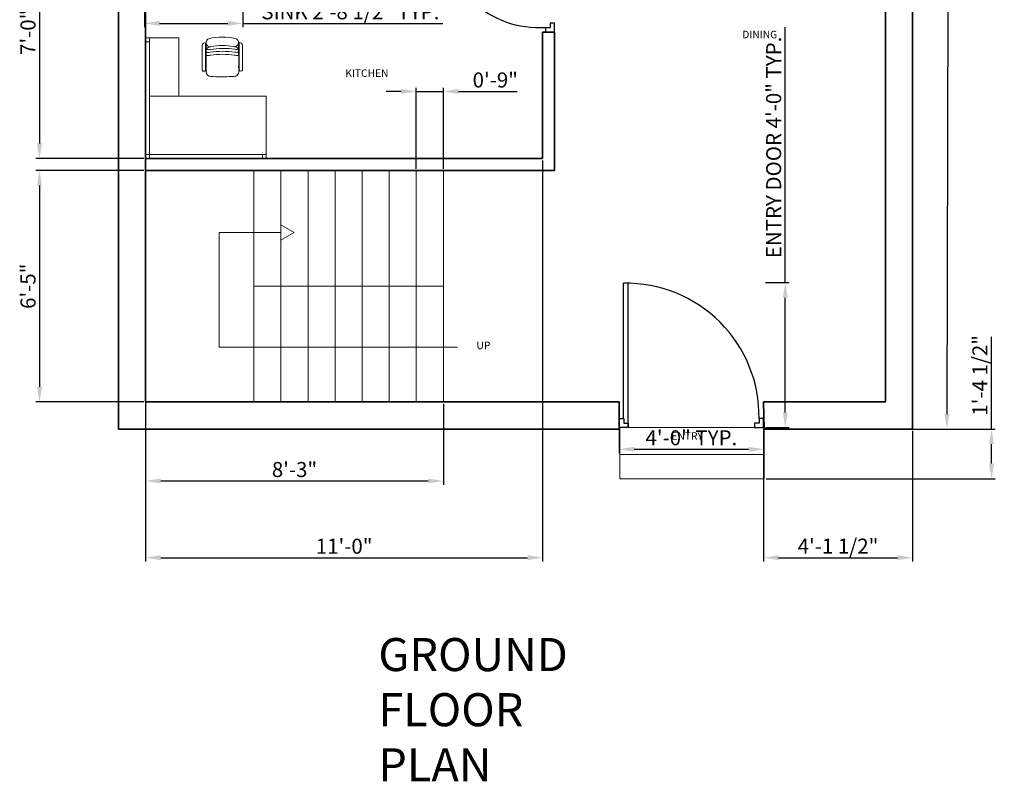
# Model space of a CAD drawing. Units: inches. Extents: x -24887 to 3061, y 1794 to 4919553.
# Tile 1 of 14: x 1576 to 1903, y 1794 to 2047. Entities that reach past the tile are written whole.
import ezdxf

# ---------------------------------------------------------------- set-up
doc = ezdxf.new("R2010")
doc.units = ezdxf.units.IN
for name, color, linetype, lineweight in [('A-ANNO-DIMS', 2, 'Continuous', 18), ('A-AREA-IDEN', 7, 'Continuous', 18), ('A-FLOR-STRS', 4, 'Continuous', 18), ('A-FURN', 8, 'Continuous', 18), ('door', 4, 'Continuous', 25), ('TEXT', 1, 'Continuous', 18), ('wall', 7, 'Continuous', 35)]:
    doc.layers.add(name, color=color, linetype=linetype, lineweight=lineweight)
doc.styles.get("Standard").update_dxf_attribs({"font": 'arial.ttf'})
doc.dimstyles.new('ISO-25', dxfattribs={"dimtxt": 5, "dimasz": 5, "dimexe": 1.25, "dimexo": 0.625, "dimtad": 1, "dimdec": 1, "dimlunit": 3, "dimtxsty": 'Standard', "dimcen": 2.5, "dimadec": 0, "dimazin": 0, "dimtfac": 1, "dimtdec": 1, "dimtmove": 0, "dimatfit": 3, "dimfxl": 1, "dimarcsym": 0})

# ---------------------------------------------------------------- blocks, each defined once
blk = doc.blocks.new('*D29')
at = {"layer": 'A-ANNO-DIMS', "color": 0, "lineweight": -2, "transparency": 16777216}
for p, q in [((1873.91, 2330.86), (1885.98, 2330.83)), ((1884.72, 2325.84), (1883.89, 1915.84)), ((1873.06, 1910.86), (1885.13, 1910.83))]:
    blk.add_line(p, q, dxfattribs=at)
at = {"layer": 'A-ANNO-DIMS', "color": 0, "transparency": 16777216}
for points in [[(1883.89, 2325.84), (1885.56, 2325.83), (1884.73, 2330.84)], [(1883.05, 1915.84), (1884.72, 1915.83), (1883.88, 1910.84)]]:
    blk.add_solid(points, dxfattribs=at)
at = {"layer": 'Defpoints', "color": 0, "transparency": 16777216}
for p in [(1873.29, 2330.86), (1872.43, 1910.86), (1883.88, 1910.84)]:
    blk.add_point(p, dxfattribs=at)
at = {"layer": 'A-ANNO-DIMS', "color": 0, "transparency": 16777216, "insert": (1881.13, 2120.84), "char_height": 5, "attachment_point": 5, "rotation": 89.8832}
blk.add_mtext("35'", dxfattribs=at)
blk = doc.blocks.new('DOOR-SINGLE-36IN')
for p, q in [((34.5, 36), (37.5, 36)), ((34.5, 34.5), (34.5, 36)), ((36, 34.5), (34.5, 34.5)), ((36, 33), (36, 34.5)), ((37.5, 33), (36, 33)), ((37.5, 36), (37.5, 33)), ((36, 3), (0, 3)), ((36, 1.5), (0, 1.5)), ((36, 1.5), (34.5, 1.5)), ((34.5, 1.5), (34.5, 0)), ((34.5, 0), (37.5, 0)), ((37.5, 3), (36, 3)), ((36, 3), (36, 1.5)), ((37.5, 0), (37.5, 3))]:
    blk.add_line(p, q)
blk.add_arc((32.32, 2.25), 32.32, 86.1244, 181.3295)
blk = doc.blocks.new('DESK-CORNER-WITH-CHAIR')
for p, q in [((0, 40.37), (40.11, 40.37)), ((0, 19.67), (0, 40.37)), ((1.29, 39.07), (1.29, 40.37)), ((38.82, 40.37), (38.82, 19.67)), ((40.11, 40.37), (40.11, 0.26)), ((0, 39.07), (40.11, 39.07)), ((38.82, 19.67), (0, 19.67)), ((29.11, 19.67), (38.82, 19.67)), ((29.11, 0.26), (29.11, 19.67)), ((38.82, 19.67), (38.82, 0.26)), ((17.49, 13.1), (18.37, 13.11)), ((7.89, 10.98), (7.93, 2.72)), ((8.97, 10.98), (9.02, 1.91)), ((9.17, 10.98), (9.17, 11.46)), ((9.17, 10.99), (9.18, 9.53)), ((10.75, 13.07), (10.91, 13.07)), ((11.62, 13.07), (10.91, 13.07)), ((19.98, 11.02), (19.97, 11.52)), ((19.98, 11.02), (19.98, 9.56)), ((20.18, 11.01), (20.22, 1.94)), ((21.26, 11.02), (21.3, 2.76)), ((9.17, 9.52), (9.22, 2.03)), ((19.99, 9.54), (20.03, 2.06)), ((40.11, 0.26), (29.11, 0.26)), ((40.11, 1.55), (38.82, 1.55))]:
    blk.add_line(p, q)
for centre, radius, start, end in [((14.78, -28.11), 41.3, 86.2317, 94.3849), ((18.38, 11.51), 1.6, 0.3083, 90.3083), ((8.43, 10.73), 0.593, 24.5958, 155.829), ((10.76, 11.47), 1.6, 90.3083, 180.3083), ((20.52, 10.77), 0.593, 204.3355, 206.5711), ((20.72, 10.77), 0.593, 24.7876, 156.0208), ((9.82, 2.64), 3.42, 74.7531, 100.4859), ((9.82, 2.64), 2.42, 74.7531, 104.4332), ((10.9, 5.33), 2.21, 220.0354, 267.4848), ((9.82, 1.7), 2.42, 74.7531, 104.4332), ((14.4, 34.16), 29.46, 262.2773, 278.3393), ((14.4, 33.22), 29.46, 262.2773, 278.3393), ((14.4, 34.16), 28.46, 262.2773, 278.3393), ((18.3, 5.37), 2.21, 273.1318, 320.9947), ((19.33, 2.69), 3.42, 78.6001, 104.4332), ((19.33, 2.69), 2.42, 73.6429, 104.4332), ((19.33, 1.75), 2.42, 73.6429, 104.4332), ((8.75, 2.68), 0.821, 177.6524, 288.8331), ((10.57, 1.77), 1.37, 80.5561, 260.4095), ((14.52, 20.73), 20.73, 258.3982, 282.2184), ((14.95, 25.37), 22.63, 259.4369, 269.1516), ((14.03, 25.37), 22.63, 271.465, 281.1797), ((18.66, 1.82), 1.37, 280.2071, 100.0605), ((20.48, 2.72), 0.821, 251.7835, 2.9643)]:
    blk.add_arc(centre, radius, start, end)
blk = doc.blocks.new('DOOR-ENTRY-48IN')
for p, q in [((1.46, 3), (1.46, 48)), ((3, 0), (3, 48)), ((0, 0), (0, 3)), ((0, 3), (1.5, 3)), ((1.5, 3), (1.5, 1.5)), ((1.5, 1.5), (3, 1.5)), ((3, 1.5), (3, 0)), ((46.5, 1.5), (45, 1.5)), ((45, 1.5), (45, 0)), ((48, 3), (46.5, 3)), ((46.5, 3), (46.5, 1.5)), ((48, 0), (48, 3)), ((3, 0), (0, 0)), ((45, 0), (48, 0))]:
    blk.add_line(p, q)
blk.add_arc((2.23, 3.73), 44.28, 359.0567, 90.9987)
blk = doc.blocks.new('*D54')
at = {"layer": 'A-ANNO-DIMS', "color": 0, "lineweight": -2, "transparency": 16777216}
for p, q in [((1617.04, 2050.09), (1617.04, 2044.56)), ((1649.71, 2050.09), (1649.71, 2044.56)), ((1622.04, 2045.81), (1644.71, 2045.81)), ((1649.71, 2045.81), (1716.31, 2045.81))]:
    blk.add_line(p, q, dxfattribs=at)
at = {"layer": 'A-ANNO-DIMS', "color": 0, "transparency": 16777216}
for points in [[(1622.04, 2046.65), (1622.04, 2044.98), (1617.04, 2045.81)], [(1644.71, 2046.65), (1644.71, 2044.98), (1649.71, 2045.81)]]:
    blk.add_solid(points, dxfattribs=at)
at = {"layer": 'Defpoints', "color": 0, "transparency": 16777216}
for p in [(1617.04, 2050.72), (1649.71, 2050.72), (1649.71, 2045.81)]:
    blk.add_point(p, dxfattribs=at)
at = {"layer": 'A-ANNO-DIMS', "color": 0, "transparency": 16777216, "insert": (1685.51, 2049.02), "char_height": 5, "attachment_point": 5}
blk.add_mtext('SINK 2\'-8 1/2" TYP.', dxfattribs=at)
blk = doc.blocks.new('*D58')
at = {"layer": 'A-ANNO-DIMS', "color": 0, "lineweight": -2, "transparency": 16777216}
for p, q in [((1830.14, 1959.56), (1830.14, 2044.54)), ((1823.53, 1959.56), (1831.39, 1959.56)), ((1830.14, 1916.35), (1830.14, 1954.56)), ((1823.53, 1911.35), (1831.39, 1911.35))]:
    blk.add_line(p, q, dxfattribs=at)
at = {"layer": 'A-ANNO-DIMS', "color": 0, "transparency": 16777216}
for points in [[(1829.31, 1954.56), (1830.97, 1954.56), (1830.14, 1959.56)], [(1829.31, 1916.35), (1830.97, 1916.35), (1830.14, 1911.35)]]:
    blk.add_solid(points, dxfattribs=at)
at = {"layer": 'Defpoints', "color": 0, "transparency": 16777216}
for p in [(1822.91, 1959.56), (1830.14, 1959.56), (1822.91, 1911.35)]:
    blk.add_point(p, dxfattribs=at)
at = {"layer": 'A-ANNO-DIMS', "color": 0, "transparency": 16777216, "insert": (1826.93, 2004.55), "char_height": 5, "attachment_point": 5, "rotation": 90}
blk.add_mtext('ENTRY DOOR 4\'-0" TYP.', dxfattribs=at)
blk = doc.blocks.new('*D59')
at = {"layer": 'A-ANNO-DIMS', "color": 0, "lineweight": -2, "transparency": 16777216}
for p, q in [((1774.91, 1910.73), (1774.91, 1902.87)), ((1822.91, 1910.73), (1822.91, 1902.87)), ((1779.91, 1904.12), (1817.91, 1904.12))]:
    blk.add_line(p, q, dxfattribs=at)
at = {"layer": 'A-ANNO-DIMS', "color": 0, "transparency": 16777216}
for points in [[(1779.91, 1904.96), (1779.91, 1903.29), (1774.91, 1904.12)], [(1817.91, 1904.96), (1817.91, 1903.29), (1822.91, 1904.12)]]:
    blk.add_solid(points, dxfattribs=at)
at = {"layer": 'Defpoints', "color": 0, "transparency": 16777216}
for p in [(1774.91, 1911.35), (1822.91, 1911.35), (1822.91, 1904.12)]:
    blk.add_point(p, dxfattribs=at)
at = {"layer": 'A-ANNO-DIMS', "color": 0, "transparency": 16777216, "insert": (1798.91, 1907.3), "char_height": 5, "attachment_point": 5}
blk.add_mtext('4\'-0" TYP.', dxfattribs=at)
blk = doc.blocks.new('*D70')
at = {"layer": 'A-ANNO-DIMS', "color": 0, "lineweight": -2, "transparency": 16777216}
for p, q in [((1617.43, 2000.23), (1617.43, 1866.79)), ((1749.43, 2000.23), (1749.43, 1866.79)), ((1622.43, 1868.04), (1744.43, 1868.04))]:
    blk.add_line(p, q, dxfattribs=at)
at = {"layer": 'A-ANNO-DIMS', "color": 0, "transparency": 16777216}
for points in [[(1622.43, 1868.88), (1622.43, 1867.21), (1617.43, 1868.04)], [(1744.43, 1868.88), (1744.43, 1867.21), (1749.43, 1868.04)]]:
    blk.add_solid(points, dxfattribs=at)
at = {"layer": 'Defpoints', "color": 0, "transparency": 16777216}
for p in [(1617.43, 2000.86), (1749.43, 2000.86), (1749.43, 1868.04)]:
    blk.add_point(p, dxfattribs=at)
at = {"layer": 'A-ANNO-DIMS', "color": 0, "transparency": 16777216, "insert": (1683.43, 1871.22), "char_height": 5, "attachment_point": 5}
blk.add_mtext('11\'-0"', dxfattribs=at)
blk = doc.blocks.new('*D73')
at = {"layer": 'A-ANNO-DIMS', "color": 0, "lineweight": -2, "transparency": 16777216}
for p, q in [((1616.81, 2084.86), (1580.88, 2084.86)), ((1582.13, 2079.86), (1582.13, 2005.86)), ((1616.81, 2000.86), (1580.88, 2000.86))]:
    blk.add_line(p, q, dxfattribs=at)
at = {"layer": 'A-ANNO-DIMS', "color": 0, "transparency": 16777216}
for points in [[(1581.3, 2079.86), (1582.96, 2079.86), (1582.13, 2084.86)], [(1581.3, 2005.86), (1582.96, 2005.86), (1582.13, 2000.86)]]:
    blk.add_solid(points, dxfattribs=at)
at = {"layer": 'Defpoints', "color": 0, "transparency": 16777216}
for p in [(1617.43, 2084.86), (1582.13, 2000.86), (1617.43, 2000.86)]:
    blk.add_point(p, dxfattribs=at)
at = {"layer": 'A-ANNO-DIMS', "color": 0, "transparency": 16777216, "insert": (1578.95, 2042.86), "char_height": 5, "attachment_point": 5, "rotation": 90}
blk.add_mtext('7\'-0"', dxfattribs=at)
blk = doc.blocks.new('*D74')
at = {"layer": 'A-ANNO-DIMS', "color": 0, "lineweight": -2, "transparency": 16777216}
for p, q in [((1616.81, 1996.86), (1580.88, 1996.86)), ((1582.13, 1991.86), (1582.13, 1924.86)), ((1616.81, 1919.86), (1580.88, 1919.86))]:
    blk.add_line(p, q, dxfattribs=at)
at = {"layer": 'A-ANNO-DIMS', "color": 0, "transparency": 16777216}
for points in [[(1581.3, 1991.86), (1582.96, 1991.86), (1582.13, 1996.86)], [(1581.3, 1924.86), (1582.96, 1924.86), (1582.13, 1919.86)]]:
    blk.add_solid(points, dxfattribs=at)
at = {"layer": 'Defpoints', "color": 0, "transparency": 16777216}
for p in [(1617.43, 1996.86), (1582.13, 1919.86), (1617.43, 1919.86)]:
    blk.add_point(p, dxfattribs=at)
at = {"layer": 'A-ANNO-DIMS', "color": 0, "transparency": 16777216, "insert": (1578.95, 1958.36), "char_height": 5, "attachment_point": 5, "rotation": 90}
blk.add_mtext('6\'-5"', dxfattribs=at)
blk = doc.blocks.new('*D75')
at = {"layer": 'A-ANNO-DIMS', "color": 0, "lineweight": -2, "transparency": 16777216}
for p, q in [((1617.43, 1919.23), (1617.43, 1892.31)), ((1716.43, 1919.23), (1716.43, 1892.31)), ((1711.43, 1893.56), (1622.43, 1893.56))]:
    blk.add_line(p, q, dxfattribs=at)
at = {"layer": 'A-ANNO-DIMS', "color": 0, "transparency": 16777216}
for points in [[(1622.43, 1894.39), (1622.43, 1892.73), (1617.43, 1893.56)], [(1711.43, 1894.39), (1711.43, 1892.73), (1716.43, 1893.56)]]:
    blk.add_solid(points, dxfattribs=at)
at = {"layer": 'Defpoints', "color": 0, "transparency": 16777216}
for p in [(1617.43, 1919.86), (1716.43, 1919.86), (1617.43, 1893.56)]:
    blk.add_point(p, dxfattribs=at)
at = {"layer": 'A-ANNO-DIMS', "color": 0, "transparency": 16777216, "insert": (1666.93, 1896.74), "char_height": 5, "attachment_point": 5}
blk.add_mtext('8\'-3"', dxfattribs=at)
blk = doc.blocks.new('*D76')
at = {"layer": 'A-ANNO-DIMS', "color": 0, "lineweight": -2, "transparency": 16777216}
for p, q in [((1822.91, 1910.23), (1822.91, 1866.79)), ((1872.43, 1910.23), (1872.43, 1866.79)), ((1827.91, 1868.04), (1867.43, 1868.04))]:
    blk.add_line(p, q, dxfattribs=at)
at = {"layer": 'A-ANNO-DIMS', "color": 0, "transparency": 16777216}
for points in [[(1827.91, 1868.88), (1827.91, 1867.21), (1822.91, 1868.04)], [(1867.43, 1868.88), (1867.43, 1867.21), (1872.43, 1868.04)]]:
    blk.add_solid(points, dxfattribs=at)
at = {"layer": 'Defpoints', "color": 0, "transparency": 16777216}
for p in [(1822.91, 1910.86), (1872.43, 1910.86), (1872.43, 1868.04)]:
    blk.add_point(p, dxfattribs=at)
at = {"layer": 'A-ANNO-DIMS', "color": 0, "transparency": 16777216, "insert": (1847.67, 1871.25), "char_height": 5, "attachment_point": 5}
blk.add_mtext('4\'-1 1/2"', dxfattribs=at)
blk = doc.blocks.new('*D77')
at = {"layer": 'A-ANNO-DIMS', "color": 0, "lineweight": -2, "transparency": 16777216}
for p, q in [((1898.73, 1910.86), (1898.73, 1941.58)), ((1823.53, 1910.86), (1899.98, 1910.86)), ((1898.73, 1899.34), (1898.73, 1905.86)), ((1823.8, 1894.34), (1899.98, 1894.34))]:
    blk.add_line(p, q, dxfattribs=at)
at = {"layer": 'A-ANNO-DIMS', "color": 0, "transparency": 16777216}
for points in [[(1897.9, 1905.86), (1899.56, 1905.86), (1898.73, 1910.86)], [(1897.9, 1899.34), (1899.56, 1899.34), (1898.73, 1894.34)]]:
    blk.add_solid(points, dxfattribs=at)
at = {"layer": 'Defpoints', "color": 0, "transparency": 16777216}
for p in [(1822.91, 1910.86), (1898.73, 1910.86), (1823.17, 1894.34)]:
    blk.add_point(p, dxfattribs=at)
at = {"layer": 'A-ANNO-DIMS', "color": 0, "transparency": 16777216, "insert": (1895.52, 1928.72), "char_height": 5, "attachment_point": 5, "rotation": 90}
blk.add_mtext('1\'-4 1/2"', dxfattribs=at)
blk = doc.blocks.new('*D78')
at = {"layer": 'A-ANNO-DIMS', "color": 0, "lineweight": -2, "transparency": 16777216}
for p, q in [((1707.43, 1997.48), (1707.43, 2024.41)), ((1716.43, 1997.48), (1716.43, 2024.41)), ((1702.43, 2023.16), (1697.43, 2023.16)), ((1707.43, 2023.16), (1716.43, 2023.16)), ((1721.43, 2023.16), (1740.97, 2023.16))]:
    blk.add_line(p, q, dxfattribs=at)
at = {"layer": 'A-ANNO-DIMS', "color": 0, "transparency": 16777216}
for points in [[(1702.43, 2023.99), (1702.43, 2022.33), (1707.43, 2023.16)], [(1721.43, 2023.99), (1721.43, 2022.33), (1716.43, 2023.16)]]:
    blk.add_solid(points, dxfattribs=at)
at = {"layer": 'Defpoints', "color": 0, "transparency": 16777216}
for p in [(1716.43, 2023.16), (1707.43, 1996.86), (1716.43, 1996.86)]:
    blk.add_point(p, dxfattribs=at)
at = {"layer": 'A-ANNO-DIMS', "color": 0, "transparency": 16777216, "insert": (1733.7, 2026.34), "char_height": 5, "attachment_point": 5}
blk.add_mtext('0\'-9"', dxfattribs=at)

msp = doc.modelspace()

# ---------------------------------------------------------------- linework, layer by layer
at = {"layer": 'A-FLOR-STRS'}
for p, q in [((1617.43, 1996.86), (1653.43, 1996.86)), ((1617.43, 1919.86), (1617.43, 1996.86)), ((1653.43, 1996.86), (1653.43, 1919.86)), ((1662.43, 1996.86), (1662.43, 1919.86)), ((1671.43, 1996.86), (1671.43, 1919.86)), ((1680.43, 1996.86), (1680.43, 1919.86)), ((1689.43, 1996.86), (1689.43, 1919.86)), ((1698.43, 1996.86), (1698.43, 1919.86)), ((1707.43, 1996.86), (1707.43, 1919.86)), ((1716.43, 1996.86), (1716.43, 1919.86)), ((1641.84, 1938.04), (1641.84, 1976.22)), ((1641.84, 1976.22), (1662.43, 1976.22)), ((1653.43, 1958.36), (1716.43, 1958.36)), ((1721.15, 1938.04), (1641.84, 1938.04)), ((1653.43, 1919.86), (1617.43, 1919.86)), ((1775.17, 1902.35), (1823.17, 1902.35))]:
    msp.add_line(p, q, dxfattribs=at)
for points in [[(1662.43, 1978.77), (1662.43, 1973.67), (1666.85, 1976.22)], [(1775.17, 1911.35), (1823.17, 1911.35), (1823.17, 1894.34), (1775.17, 1894.34)]]:
    msp.add_lwpolyline(points, close=True, dxfattribs=at)
at = {"layer": 'wall'}
for p, q in [((1608.43, 2330.86), (1608.43, 1910.86)), ((1872.43, 1910.86), (1872.43, 2330.86)), ((1617.43, 2321.86), (1617.43, 1919.86)), ((1863.43, 1919.86), (1863.43, 2321.86)), ((1749.43, 2042.86), (1753.43, 2042.86)), ((1749.43, 2042.86), (1749.43, 2000.86)), ((1753.43, 2042.86), (1753.43, 1996.86)), ((1749.43, 2000.86), (1617.43, 2000.86)), ((1753.43, 1996.86), (1617.43, 1996.86)), ((1617.43, 1919.86), (1774.91, 1919.86)), ((1774.91, 1919.86), (1774.91, 1910.86)), ((1822.91, 1919.86), (1863.43, 1919.86)), ((1822.91, 1919.86), (1823.17, 1910.86)), ((1608.43, 1910.86), (1774.91, 1910.86)), ((1822.91, 1910.86), (1872.43, 1910.86))]:
    msp.add_line(p, q, dxfattribs=at)

# ---------------------------------------------------------------- block references
at = {"layer": 'A-FURN', "rotation": 180}
msp.add_blockref('DESK-CORNER-WITH-CHAIR', (1657.54, 2041.23), dxfattribs=at)
at = {"layer": 'door', "extrusion": (0, 0, -1), "zscale": -1, "rotation": 180}
msp.add_blockref('DOOR-SINGLE-36IN', (-1715.93, 2078.88), dxfattribs=at)
at = {"layer": 'door'}
msp.add_blockref('DOOR-ENTRY-48IN', (1774.91, 1911.35), dxfattribs=at)

# ---------------------------------------------------------------- texts
at = {"layer": 'A-AREA-IDEN', "char_height": 2.5, "attachment_point": 1}
for s, insert in [('DINING', (1815.84, 2043.36)), ('KITCHEN', (1683.81, 2030.52))]:
    msp.add_mtext_dynamic_manual_height_columns(s, width=34.2323, gutter_width=12.5, heights=[0], dxfattribs=dict(at, insert=insert))
at = {"layer": 'TEXT', "attachment_point": 1}
for s, insert, char_height in [('UP', (1727.45, 1939.92), 2.5), ('ENTRY', (1792.28, 1909.8), 2.5), ('GROUND FLOOR PLAN', (1694.81, 1841.32), 11)]:
    msp.add_mtext_dynamic_manual_height_columns(s, width=34.2323, gutter_width=12.5, heights=[0], dxfattribs=dict(at, insert=insert, char_height=char_height))

# ---------------------------------------------------------------- dimensions: what is measured, and where the dimension line sits
at = {"layer": 'A-ANNO-DIMS'}
dim = msp.add_aligned_dim(p1=(1873.29, 2330.86), p2=(1872.43, 1910.86), distance=11.45, dimstyle='ISO-25', override={"dimclrd": 0, "dimclre": 0, "dimclrt": 0}, dxfattribs=at)
dim.commit()
dim.dimension.update_dxf_attribs({"geometry": '*D29', "text_midpoint": (1881.13, 2120.84)})
for base, p1, p2, angle, picture, middle in [((1582.13, 2000.86), (1617.43, 2084.86), (1617.43, 2000.86), 90, '*D73', (1578.95, 2042.86)), ((1582.13, 1919.86), (1617.43, 1996.86), (1617.43, 1919.86), 90, '*D74', (1578.95, 1958.36)), ((1898.73, 1910.86), (1823.17, 1894.34), (1822.91, 1910.86), 90, '*D77', (1895.52, 1928.72)), ((1617.43, 1893.56), (1716.43, 1919.86), (1617.43, 1919.86), 180, '*D75', (1666.93, 1896.74))]:
    dim = msp.add_linear_dim(base=base, p1=p1, p2=p2, angle=angle, dimstyle='ISO-25', override={"dimdec": 1, "dimlfac": 1, "dimrnd": 0, "dimzin": 1, "dimdsep": 46, "dimlunit": 4, "dimfrac": 2}, dxfattribs=at)
    dim.commit()
    dim.dimension.update_dxf_attribs({"geometry": picture, "text_midpoint": middle})
for base, p1, p2, text, picture, middle in [((1649.71, 2045.81), (1617.04, 2050.72), (1649.71, 2050.72), 'SINK <> TYP.', '*D54', (1685.51, 2049.02)), ((1822.91, 1904.12), (1774.91, 1911.35), (1822.91, 1911.35), '<> TYP.', '*D59', (1798.91, 1907.3))]:
    dim = msp.add_linear_dim(base=base, p1=p1, p2=p2, text=text, dimstyle='ISO-25', override={"dimdec": 1, "dimlfac": 1, "dimrnd": 0, "dimzin": 1, "dimdsep": 46, "dimlunit": 4, "dimfrac": 2}, dxfattribs=at)
    dim.commit()
    dim.dimension.update_dxf_attribs({"geometry": picture, "text_midpoint": middle})
dim = msp.add_linear_dim(base=(1830.14, 1959.56), p1=(1822.91, 1911.35), p2=(1822.91, 1959.56), angle=90, text='ENTRY DOOR <> TYP.', dimstyle='ISO-25', override={"dimdec": 1, "dimlfac": 1, "dimrnd": 0, "dimzin": 1, "dimdsep": 46, "dimlunit": 4, "dimfrac": 2}, dxfattribs=at)
dim.commit()
dim.dimension.update_dxf_attribs({"geometry": '*D58', "text_midpoint": (1826.93, 2004.55)})
for base, p1, p2, picture, middle in [((1716.43, 2023.16), (1707.43, 1996.86), (1716.43, 1996.86), '*D78', (1733.7, 2026.34)), ((1749.43, 1868.04), (1617.43, 2000.86), (1749.43, 2000.86), '*D70', (1683.43, 1871.22)), ((1872.43, 1868.04), (1822.91, 1910.86), (1872.43, 1910.86), '*D76', (1847.67, 1871.25))]:
    dim = msp.add_linear_dim(base=base, p1=p1, p2=p2, dimstyle='ISO-25', override={"dimdec": 1, "dimlfac": 1, "dimrnd": 0, "dimzin": 1, "dimdsep": 46, "dimlunit": 4, "dimfrac": 2}, dxfattribs=at)
    dim.commit()
    dim.dimension.update_dxf_attribs({"geometry": picture, "text_midpoint": middle})

doc.saveas('drawing.dxf')
